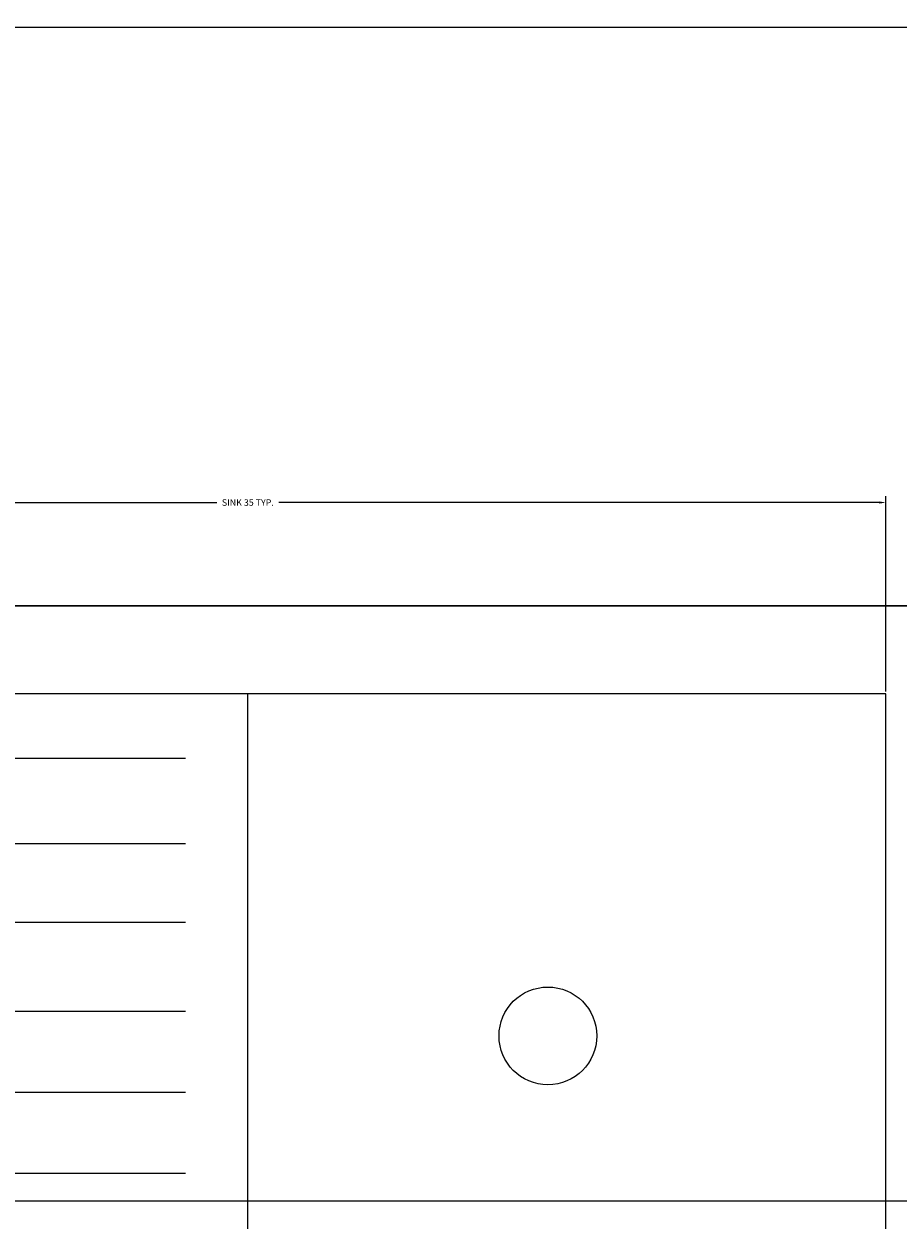
# Model space of a CAD drawing. Units: inches. Extents: x 1998 to 2588, y 1139 to 1977.
# Tile 18 of 134: x 2171 to 2195, y 1596 to 1629. Entities that reach past the tile are written whole.
import ezdxf

# ---------------------------------------------------------------- set-up
doc = ezdxf.new("R2010")
doc.units = ezdxf.units.IN
for name, color, linetype, lineweight in [('A-ANNO-DIMS', 2, 'Continuous', 18), ('A-FLOR-CASE', 32, 'Continuous', 25), ('A-FLOR-FIXT', 9, 'Continuous', 18)]:
    doc.layers.add(name, color=color, linetype=linetype, lineweight=lineweight)
doc.styles.get("Standard").update_dxf_attribs({"font": 'arial.ttf'})
doc.dimstyles.get("Standard").update_dxf_attribs({"dimtxt": 0.18, "dimasz": 0.18, "dimexe": 0.18, "dimexo": 0.0625, "dimgap": 0.09, "dimtad": 0, "dimtih": 1, "dimtoh": 1, "dimdec": 4, "dimzin": 0, "dimdsep": 46, "dimtxsty": 'Standard', "dimcen": 0.09, "dimadec": 0, "dimazin": 0, "dimtfac": 1, "dimtdec": 4, "dimtofl": 0, "dimtmove": 0, "dimatfit": 3, "dimfxl": 1, "dimtolj": 1, "dimtzin": 0, "dimarcsym": 0})

# ---------------------------------------------------------------- blocks, each defined once
blk = doc.blocks.new('SINK-WITH-DRAINBOARD')
for p, q in [((17.653, 0), (17.653, 19.174)), ((15.925, 17.391), (2.574, 17.391)), ((15.925, 15.023), (2.574, 15.023)), ((15.925, 12.848), (2.574, 12.848)), ((15.925, 10.383), (2.574, 10.383)), ((15.925, 8.143), (2.574, 8.143)), ((15.925, 5.899), (2.574, 5.899)), ((15.925, 3.752), (2.574, 3.752))]:
    blk.add_line(p, q)
blk.add_lwpolyline([(35.306, 19.174), (0, 19.174), (0, 0), (35.306, 0)], close=True)
blk.add_circle((25.956, 9.71), 1.353)
blk = doc.blocks.new('*D19')
at = {"layer": 'A-ANNO-DIMS', "color": 0, "lineweight": -2, "transparency": 16777216}
for p, q in [((2159.737, 1610.356), (2159.737, 1615.769)), ((2195.043, 1610.356), (2195.043, 1615.769)), ((2159.917, 1615.589), (2176.534, 1615.589)), ((2194.863, 1615.589), (2178.246, 1615.589))]:
    blk.add_line(p, q, dxfattribs=at)
at = {"layer": 'A-ANNO-DIMS', "color": 0, "transparency": 16777216}
for points in [[(2159.917, 1615.619), (2159.917, 1615.559), (2159.737, 1615.589)], [(2194.863, 1615.619), (2194.863, 1615.559), (2195.043, 1615.589)]]:
    blk.add_solid(points, dxfattribs=at)
at = {"layer": 'Defpoints', "color": 0, "transparency": 16777216}
for p in [(2195.043, 1615.589), (2159.737, 1610.293), (2195.043, 1610.293)]:
    blk.add_point(p, dxfattribs=at)
at = {"layer": 'A-ANNO-DIMS', "color": 0, "transparency": 16777216, "insert": (2177.39, 1615.589), "char_height": 0.18, "attachment_point": 5}
blk.add_mtext('\\A1;SINK 35 TYP.', dxfattribs=at)
blk = doc.blocks.new('*D30')
at = {"layer": 'A-ANNO-DIMS', "color": 0, "lineweight": -2, "transparency": 16777216}
for p, q in [((2407.91, 1636.732), (1997.843, 1636.732)), ((1998.023, 1636.552), (1998.023, 1615.913)), ((1998.023, 1594.912), (1998.023, 1615.552)), ((2407.91, 1594.732), (1997.843, 1594.732))]:
    blk.add_line(p, q, dxfattribs=at)
at = {"layer": 'A-ANNO-DIMS', "color": 0, "transparency": 16777216}
for points in [[(1997.993, 1636.552), (1998.053, 1636.552), (1998.023, 1636.732)], [(1997.993, 1594.912), (1998.053, 1594.912), (1998.023, 1594.732)]]:
    blk.add_solid(points, dxfattribs=at)
at = {"layer": 'Defpoints', "color": 0, "transparency": 16777216}
for p in [(1998.023, 1636.732), (2407.973, 1636.732), (2407.973, 1594.732)]:
    blk.add_point(p, dxfattribs=at)
at = {"layer": 'A-ANNO-DIMS', "color": 0, "transparency": 16777216, "insert": (1998.023, 1615.732), "char_height": 0.18, "attachment_point": 5}
blk.add_mtext('\\A1;42', dxfattribs=at)
blk = doc.blocks.new('*D37')
at = {"layer": 'A-ANNO-DIMS', "color": 0, "lineweight": -2, "transparency": 16777216}
for p, q in [((2148.455, 1612.795), (2148.455, 1977.362)), ((2148.635, 1977.182), (2172.73, 1977.182)), ((2197.27, 1977.182), (2173.175, 1977.182)), ((2197.45, 1612.795), (2197.45, 1977.362))]:
    blk.add_line(p, q, dxfattribs=at)
at = {"layer": 'A-ANNO-DIMS', "color": 0, "transparency": 16777216}
for points in [[(2148.635, 1977.212), (2148.635, 1977.152), (2148.455, 1977.182)], [(2197.27, 1977.212), (2197.27, 1977.152), (2197.45, 1977.182)]]:
    blk.add_solid(points, dxfattribs=at)
at = {"layer": 'Defpoints', "color": 0, "transparency": 16777216}
for p in [(2197.45, 1977.182), (2148.455, 1612.732), (2197.45, 1612.732)]:
    blk.add_point(p, dxfattribs=at)
at = {"layer": 'A-ANNO-DIMS', "color": 0, "transparency": 16777216, "insert": (2172.952, 1977.182), "char_height": 0.18, "attachment_point": 5}
blk.add_mtext('\\A1;49', dxfattribs=at)
blk = doc.blocks.new('*D38')
at = {"layer": 'A-ANNO-DIMS', "color": 0, "lineweight": -2, "transparency": 16777216}
for p, q in [((2197.387, 1663.247), (1997.843, 1663.247)), ((1998.023, 1663.067), (1998.023, 1638.171)), ((1998.023, 1612.912), (1998.023, 1637.808)), ((2197.387, 1612.732), (1997.843, 1612.732))]:
    blk.add_line(p, q, dxfattribs=at)
at = {"layer": 'A-ANNO-DIMS', "color": 0, "transparency": 16777216}
for points in [[(1997.993, 1663.067), (1998.053, 1663.067), (1998.023, 1663.247)], [(1997.993, 1612.912), (1998.053, 1612.912), (1998.023, 1612.732)]]:
    blk.add_solid(points, dxfattribs=at)
at = {"layer": 'Defpoints', "color": 0, "transparency": 16777216}
for p in [(1998.023, 1663.247), (2197.45, 1663.247), (2197.45, 1612.732)]:
    blk.add_point(p, dxfattribs=at)
at = {"layer": 'A-ANNO-DIMS', "color": 0, "transparency": 16777216, "insert": (1998.023, 1637.99), "char_height": 0.18, "attachment_point": 5}
blk.add_mtext('\\A1;50.51', dxfattribs=at)
blk = doc.blocks.new('*D39')
at = {"layer": 'A-ANNO-DIMS', "color": 0, "lineweight": -2, "transparency": 16777216}
for p, q in [((2115.035, 1628.742), (2588.309, 1628.742)), ((2588.129, 1628.562), (2588.129, 1612.685)), ((2588.129, 1596.444), (2588.129, 1612.321)), ((2115.035, 1596.264), (2588.309, 1596.264))]:
    blk.add_line(p, q, dxfattribs=at)
at = {"layer": 'A-ANNO-DIMS', "color": 0, "transparency": 16777216}
for points in [[(2588.099, 1628.562), (2588.159, 1628.562), (2588.129, 1628.742)], [(2588.099, 1596.444), (2588.159, 1596.444), (2588.129, 1596.264)]]:
    blk.add_solid(points, dxfattribs=at)
at = {"layer": 'Defpoints', "color": 0, "transparency": 16777216}
for p in [(2114.973, 1628.742), (2588.129, 1628.742), (2114.973, 1596.264)]:
    blk.add_point(p, dxfattribs=at)
at = {"layer": 'A-ANNO-DIMS', "color": 0, "transparency": 16777216, "insert": (2588.129, 1612.503), "char_height": 0.18, "attachment_point": 5}
blk.add_mtext('\\A1;32.48', dxfattribs=at)

msp = doc.modelspace()

# ---------------------------------------------------------------- linework, layer by layer
at = {"layer": 'A-FLOR-CASE'}
msp.add_line((2148.4548, 1612.7324), (2197.4499, 1612.7324), dxfattribs=at)

# ---------------------------------------------------------------- block references
at = {"layer": 'A-FLOR-FIXT'}
msp.add_blockref('SINK-WITH-DRAINBOARD', (2159.737, 1591.119), dxfattribs=at)

# ---------------------------------------------------------------- dimensions: what is measured, and where the dimension line sits
at = {"layer": 'A-ANNO-DIMS'}
dim = msp.add_linear_dim(base=(2197.4499, 1977.1824), p1=(2148.4548, 1612.7324), p2=(2197.4499, 1612.7324), dimstyle='Standard', override={"dimdec": 0, "dimlfac": 1, "dimrnd": 0, "dimzin": 0, "dimdsep": 46, "dimlunit": 2}, dxfattribs=at)
dim.commit()
dim.dimension.update_dxf_attribs({"geometry": '*D37', "text_midpoint": (2172.9524, 1977.1824)})
for base, p1, p2, override, picture, middle in [((1998.0229, 1663.2466), (2197.4499, 1612.7324), (2197.4499, 1663.2466), {"dimdec": 2, "dimlfac": 1, "dimrnd": 0, "dimzin": 0, "dimdsep": 46, "dimlunit": 2}, '*D38', (1998.0229, 1637.9895)), ((1998.0229, 1636.7324), (2407.9729, 1594.7324), (2407.9729, 1636.7324), {"dimdec": 0, "dimlfac": 1, "dimrnd": 0, "dimzin": 0, "dimdsep": 46, "dimlunit": 2}, '*D30', (1998.0229, 1615.7324)), ((2588.1286, 1628.7416), (2114.9729, 1596.2642), (2114.9729, 1628.7416), {"dimdec": 2, "dimlfac": 1, "dimrnd": 0, "dimzin": 0, "dimdsep": 46, "dimlunit": 2}, '*D39', (2588.1286, 1612.5029))]:
    dim = msp.add_linear_dim(base=base, p1=p1, p2=p2, angle=90, dimstyle='Standard', override=override, dxfattribs=at)
    dim.commit()
    dim.dimension.update_dxf_attribs({"geometry": picture, "text_midpoint": middle})
dim = msp.add_linear_dim(base=(2195.0425, 1615.5894), p1=(2159.7366, 1610.2935), p2=(2195.0425, 1610.2935), text='SINK <> TYP.', dimstyle='Standard', override={"dimdec": 0, "dimlfac": 1, "dimrnd": 0, "dimzin": 0, "dimdsep": 46, "dimlunit": 2}, dxfattribs=at)
dim.commit()
dim.dimension.update_dxf_attribs({"geometry": '*D19', "text_midpoint": (2177.3896, 1615.5894)})

doc.saveas('drawing.dxf')
